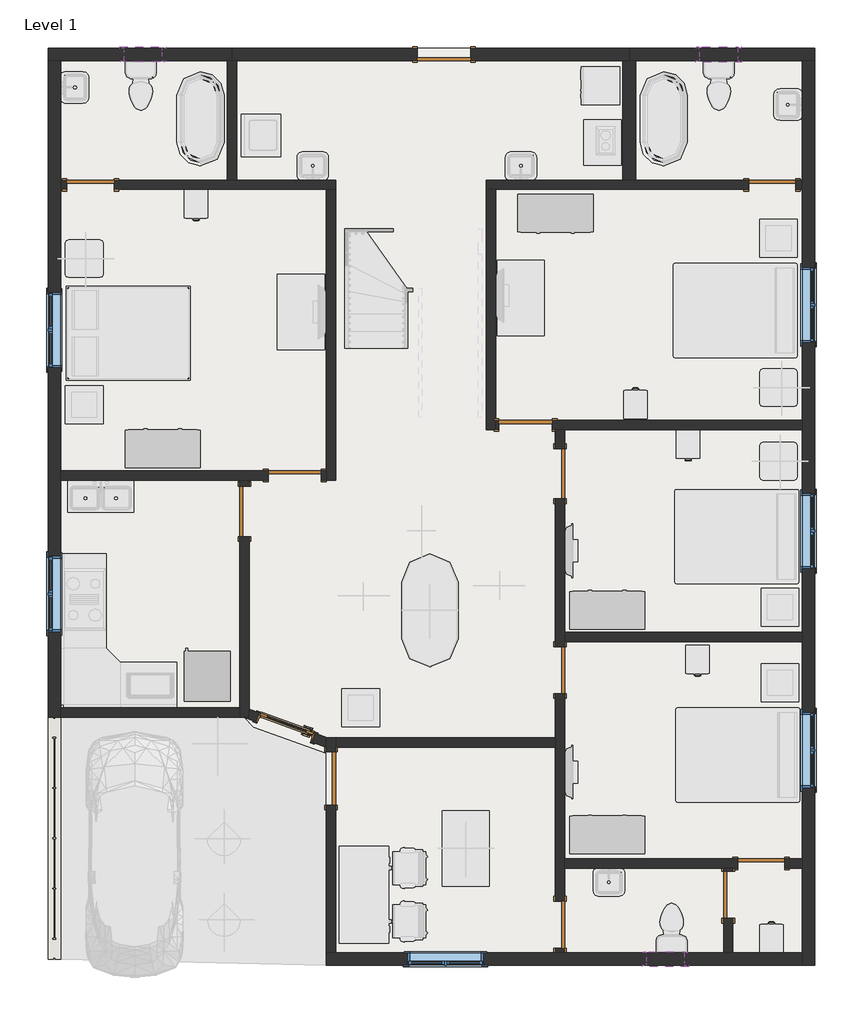
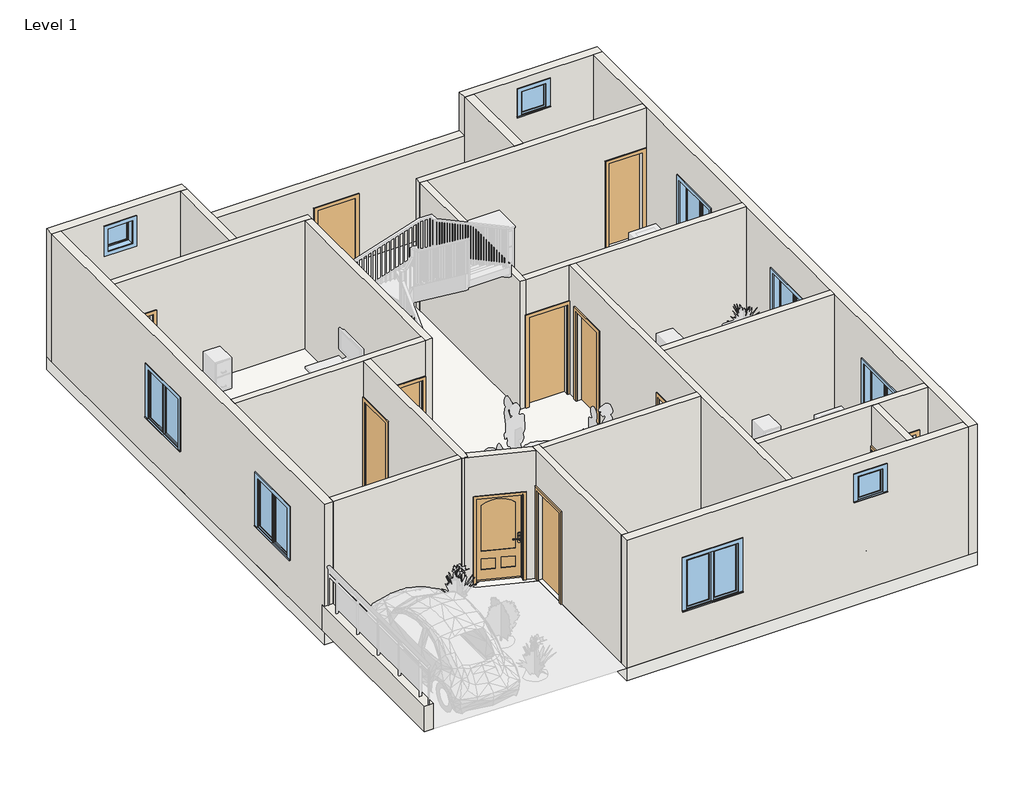
# One storey, part 1 of 3: 24 walls, 13 doors, 9 windows, 1 slab.
"""IFC4 building model written with IfcOpenShell, lengths in millimetres."""

from ifc_helpers import new_model, si_unit, frame, origin, origin_with_axes, place, context, project, spatial, polyline, outline, extrude, faceted_brep, transform, mapped, element, save
from components import door_808aeb8e, door_255cab33, door_059fdd7e, door_377e7377, door_bb092f7c, door_3e6ab620, door_b6e9fca3, door_99d96fc5, window_0862ab64, window_e41d21a6

model = new_model("IFC4")

# Units and contexts
model_context = context("Model", 3, world=origin())
ifc_project = project(units=[si_unit("LENGTHUNIT", "METRE", prefix="MILLI")], contexts=[model_context])

# Site, building, storey
site = spatial("IfcSite", under=ifc_project)
building = spatial("IfcBuilding", under=site)
storey = spatial("IfcBuildingStorey", under=building, Name="Level 1", Elevation=0.0)

# Doors
placement = place(None, origin())
door_shape = door_808aeb8e(model_context)
element("IfcDoor", 1, ObjectType="36\" x 80\"", at=placement, inside=storey, context=model_context, shape_type="MappedRepresentation", body=[
    mapped(door_shape, transform((-11135.4937633, 2943.8996558, 0.0), x_axis=(0.9396926207859074, -0.3420201433256715, 0.0), y_axis=(0.3420201433256715, 0.9396926207859074, 0.0), z_axis=(0.0, 0.0, 1.0))),
])
door_2_shape = door_255cab33(model_context)
element("IfcDoor", 2, ObjectType="Single-Flush : 30\" x 80\"", at=placement, inside=storey, context=model_context, shape_type="MappedRepresentation", body=[
    mapped(door_2_shape, transform((-14290.4744419, 11717.2452409, 0.0), x_axis=(-1.0, 0.0, 0.0), y_axis=(0.0, -1.0, 0.0), z_axis=(0.0, 0.0, 1.0))),
])
element("IfcDoor", 3, ObjectType="Single-Flush : 30\" x 80\"", at=placement, inside=storey, context=model_context, shape_type="MappedRepresentation", body=[
    mapped(door_2_shape, transform((-6695.8744419, 3868.6452409, 0.0), x_axis=(0.0, 1.0, 0.0), y_axis=(-1.0, 0.0, 0.0), z_axis=(0.0, 0.0, 1.0))),
])
element("IfcDoor", 4, ObjectType="Single-Flush : 30\" x 80\"", at=placement, inside=storey, context=model_context, shape_type="MappedRepresentation", body=[
    mapped(door_2_shape, transform((-3444.6744419, 744.4452409, 0.0), x_axis=(-1.0, 0.0, 0.0), y_axis=(0.0, -1.0, 0.0), z_axis=(0.0, 0.0, 1.0))),
])
door_3_shape = door_059fdd7e(model_context)
element("IfcDoor", 5, ObjectType="Single-Flush : 30\" x 80\"", at=placement, inside=storey, context=model_context, shape_type="MappedRepresentation", body=[
    mapped(door_3_shape, transform((-3266.8744419, 11717.2452409, 0.0), x_axis=(1.0, 0.0, 0.0), y_axis=(0.0, 1.0, 0.0), z_axis=(0.0, 0.0, 1.0))),
])
element("IfcDoor", 6, ObjectType="Single-Flush : 30\" x 80\"", at=placement, inside=storey, context=model_context, shape_type="MappedRepresentation", body=[
    mapped(door_3_shape, transform((-6695.8744419, -246.1547591, 0.0), x_axis=(0.0, -1.0, 0.0), y_axis=(1.0, 0.0, 0.0), z_axis=(0.0, 0.0, 1.0))),
])
element("IfcDoor", 7, ObjectType="Single-Flush : 30\" x 80\"", at=placement, inside=storey, context=model_context, shape_type="MappedRepresentation", body=[
    mapped(door_3_shape, transform((-3978.0744419, 236.4452409, 0.0), x_axis=(0.0, 1.0, 0.0), y_axis=(-1.0, 0.0, 0.0), z_axis=(0.0, 0.0, 1.0))),
])
door_4_shape = door_377e7377(model_context)
element("IfcDoor", 8, ObjectType="Single-Flush : 32\" x 84\"", at=placement, inside=storey, context=model_context, shape_type="MappedRepresentation", body=[
    mapped(door_4_shape, transform((-11801.2744419, 6434.0452409, 0.0), x_axis=(0.0, 1.0, 0.0), y_axis=(-1.0, 0.0, 0.0), z_axis=(0.0, 0.0, 1.0))),
])
door_5_shape = door_bb092f7c(model_context)
element("IfcDoor", 9, ObjectType="Single-Flush : 32\" x 84\"", at=placement, inside=storey, context=model_context, shape_type="MappedRepresentation", body=[
    mapped(door_5_shape, transform((-6695.8744419, 7043.6452409, 0.0), x_axis=(0.0, 1.0, 0.0), y_axis=(-1.0, 0.0, 0.0), z_axis=(0.0, 0.0, 1.0))),
])
door_6_shape = door_3e6ab620(model_context)
element("IfcDoor", 10, ObjectType="Single-Flush : 34\" x 60\"", at=placement, inside=storey, context=model_context, shape_type="MappedRepresentation", body=[
    mapped(door_6_shape, transform((-8575.4744419, 13825.4452409, 0.0), x_axis=(-1.0, 0.0, 0.0), y_axis=(0.0, -1.0, 0.0), z_axis=(0.0, 0.0, 1.0))),
])
door_7_shape = door_b6e9fca3(model_context)
element("IfcDoor", 11, ObjectType="Single-Flush : 34\" x 84\"", at=placement, inside=storey, context=model_context, shape_type="MappedRepresentation", body=[
    mapped(door_7_shape, transform((-10988.4744419, 7018.2452409, 0.0), x_axis=(1.0, 0.0, 0.0), y_axis=(0.0, 1.0, 0.0), z_axis=(0.0, 0.0, 1.0))),
])
door_8_shape = door_99d96fc5(model_context)
element("IfcDoor", 12, ObjectType="Single-Flush : 34\" x 84\"", at=placement, inside=storey, context=model_context, shape_type="MappedRepresentation", body=[
    mapped(door_8_shape, transform((-7254.6744419, 7831.0452409, 0.0), x_axis=(-1.0, 0.0, 0.0), y_axis=(0.0, -1.0, 0.0), z_axis=(0.0, 0.0, 1.0))),
])
element("IfcDoor", 13, ObjectType="Single-Flush : 34\" x 84\"", at=placement, inside=storey, context=model_context, shape_type="MappedRepresentation", body=[
    mapped(door_8_shape, transform((-10404.2744419, 2116.0452409, 0.0), x_axis=(0.0, 1.0, 0.0), y_axis=(-1.0, 0.0, 0.0), z_axis=(0.0, 0.0, 1.0))),
])

# Slab
element("IfcSlab", 14, ObjectType="Generic - 12\"", at=placement, inside=storey, context=model_context, shape_type="SweptSolid", body=[
    extrude(outline(polyline([(-2581.0744419, 13927.0452409), (-2581.0744419, -906.5547591), (-10480.4744419, -906.5547591), (-10480.4744419, 2522.4452409), (-11647.819555, 2947.3241152), (-11807.1406807, 3106.6452409), (-14976.2744419, 3106.6452409), (-14976.2744419, 13927.0452409), (-2581.0744419, 13927.0452409)])), frame((0.0, 0.0, -304.8), z_axis=(0.0, 0.0, 1.0), x_axis=(1.0, 0.0, 0.0)), (0.0, 0.0, 1.0), 304.8),
])

# Walls
element("IfcWall", 15, ObjectType="Generic - 2'", at=placement, inside=storey, context=model_context, shape_type="Brep", body=[
    faceted_brep([(-14773.0744419, -804.9547591, 0.0), (-14773.0744419, 3106.6452409, 0.0), (-14773.0744419, 3182.8452409, 0.0), (-14773.0744419, 3182.8452409, 609.6), (-14773.0744419, -804.9547591, 609.6), (-14976.2744419, -804.9547591, 0.0), (-14976.2744419, -804.9547591, 609.6), (-14976.2744419, 3182.8452409, 609.6), (-14976.2744419, 3182.8452409, 0.0)], [[[0, 1, 2, 3, 4]], [[5, 6, 7, 8]], [[2, 1, 0, 5, 8]], [[3, 2, 8, 7]], [[4, 3, 7, 6]], [[0, 4, 6, 5]]]),
])
element("IfcWall", 16, ObjectType="Generic - 8\"", at=placement, inside=storey, context=model_context, shape_type="Brep", body=[
    faceted_brep([(-14976.2744419, 13723.8452409, 0.0), (-14773.0744419, 13723.8452409, 0.0), (-12080.6744419, 13723.8452409, 0.0), (-12004.4744419, 13723.8452409, 0.0), (-12004.4744419, 13723.8452409, 2133.6), (-11928.2744419, 13723.8452409, 2133.6), (-11928.2744419, 13723.8452409, 3048.0), (-12080.6744419, 13723.8452409, 3048.0), (-14773.0744419, 13723.8452409, 3048.0), (-14976.2744419, 13723.8452409, 3048.0), (-13134.7744419, 13723.8452409, 2768.6), (-13134.7744419, 13723.8452409, 2159.0), (-13744.3744419, 13723.8452409, 2159.0), (-13744.3744419, 13723.8452409, 2768.6), (-14976.2744419, 13927.0452409, 0.0), (-14976.2744419, 13927.0452409, 3048.0), (-11928.2744419, 13927.0452409, 3048.0), (-11928.2744419, 13927.0452409, 2133.6), (-12004.4744419, 13927.0452409, 2133.6), (-12004.4744419, 13927.0452409, 0.0), (-13134.7744419, 13927.0452409, 2768.6), (-13744.3744419, 13927.0452409, 2768.6), (-13744.3744419, 13927.0452409, 2159.0), (-13134.7744419, 13927.0452409, 2159.0)], [[[0, 1, 2, 3, 4, 5, 6, 7, 8, 9], [10, 11, 12, 13]], [[14, 15, 16, 17, 18, 19], [20, 21, 22, 23]], [[3, 2, 1, 0, 14, 19]], [[0, 9, 15, 14]], [[11, 10, 20, 23]], [[12, 11, 23, 22]], [[13, 12, 22, 21]], [[10, 13, 21, 20]], [[4, 3, 19, 18]], [[17, 5, 4, 18]], [[6, 5, 17, 16]], [[9, 8, 7, 6, 16, 15]]]),
])
element("IfcWall", 17, ObjectType="Generic - 8\"", at=placement, inside=storey, context=model_context, shape_type="Brep", body=[
    faceted_brep([(-2784.2744419, 13723.8452409, 0.0), (-2784.2744419, 11793.4452409, 0.0), (-2784.2744419, 11641.0452409, 0.0), (-2784.2744419, 7907.2452409, 0.0), (-2784.2744419, 7754.8452409, 0.0), (-2784.2744419, 4478.2452409, 0.0), (-2784.2744419, 4325.8452409, 0.0), (-2784.2744419, 820.6452409, 0.0), (-2784.2744419, 668.2452409, 0.0), (-2784.2744419, -703.3547591, 0.0), (-2784.2744419, -906.5547591, 0.0), (-2784.2744419, -906.5547591, 3048.0), (-2784.2744419, -703.3547591, 3048.0), (-2784.2744419, 668.2452409, 3048.0), (-2784.2744419, 820.6452409, 3048.0), (-2784.2744419, 4325.8452409, 3048.0), (-2784.2744419, 4478.2452409, 3048.0), (-2784.2744419, 7754.8452409, 3048.0), (-2784.2744419, 7907.2452409, 3048.0), (-2784.2744419, 11641.0452409, 3048.0), (-2784.2744419, 11793.4452409, 3048.0), (-2784.2744419, 13723.8452409, 3048.0), (-2784.2744419, 1963.6452409, 2133.6), (-2784.2744419, 1963.6452409, 914.4), (-2784.2744419, 3182.8452409, 914.4), (-2784.2744419, 3182.8452409, 2133.6), (-2784.2744419, 5506.9452409, 2133.6), (-2784.2744419, 5506.9452409, 914.4), (-2784.2744419, 6726.1452409, 914.4), (-2784.2744419, 6726.1452409, 2133.6), (-2784.2744419, 9164.5452409, 2133.6), (-2784.2744419, 9164.5452409, 914.4), (-2784.2744419, 10383.7452409, 914.4), (-2784.2744419, 10383.7452409, 2133.6), (-2581.0744419, 13723.8452409, 0.0), (-2581.0744419, 13723.8452409, 3048.0), (-2581.0744419, -906.5547591, 3048.0), (-2581.0744419, -906.5547591, 0.0), (-2581.0744419, 1963.6452409, 2133.6), (-2581.0744419, 3182.8452409, 2133.6), (-2581.0744419, 3182.8452409, 914.4), (-2581.0744419, 1963.6452409, 914.4), (-2581.0744419, 5506.9452409, 2133.6), (-2581.0744419, 6726.1452409, 2133.6), (-2581.0744419, 6726.1452409, 914.4), (-2581.0744419, 5506.9452409, 914.4), (-2581.0744419, 9164.5452409, 2133.6), (-2581.0744419, 10383.7452409, 2133.6), (-2581.0744419, 10383.7452409, 914.4), (-2581.0744419, 9164.5452409, 914.4)], [[[0, 1, 2, 3, 4, 5, 6, 7, 8, 9, 10, 11, 12, 13, 14, 15, 16, 17, 18, 19, 20, 21], [22, 23, 24, 25], [26, 27, 28, 29], [30, 31, 32, 33]], [[34, 35, 36, 37], [38, 39, 40, 41], [42, 43, 44, 45], [46, 47, 48, 49]], [[10, 9, 8, 7, 6, 5, 4, 3, 2, 1, 0, 34, 37]], [[0, 21, 35, 34]], [[11, 10, 37, 36]], [[23, 22, 38, 41]], [[24, 23, 41, 40]], [[25, 24, 40, 39]], [[22, 25, 39, 38]], [[27, 26, 42, 45]], [[28, 27, 45, 44]], [[29, 28, 44, 43]], [[26, 29, 43, 42]], [[31, 30, 46, 49]], [[32, 31, 49, 48]], [[33, 32, 48, 47]], [[30, 33, 47, 46]], [[21, 20, 19, 18, 17, 16, 15, 14, 13, 12, 11, 36, 35]]]),
])
element("IfcWall", 18, ObjectType="Generic - 8\"", at=placement, inside=storey, context=model_context, shape_type="Brep", body=[
    faceted_brep([(-2784.2744419, -703.3547591, 0.0), (-3901.8744419, -703.3547591, 0.0), (-4054.2744419, -703.3547591, 0.0), (-6619.6744419, -703.3547591, 0.0), (-6772.0744419, -703.3547591, 0.0), (-10328.0744419, -703.3547591, 0.0), (-10480.4744419, -703.3547591, 0.0), (-10480.4744419, -703.3547591, 3048.0), (-10328.0744419, -703.3547591, 3048.0), (-6772.0744419, -703.3547591, 3048.0), (-6619.6744419, -703.3547591, 3048.0), (-4054.2744419, -703.3547591, 3048.0), (-3901.8744419, -703.3547591, 3048.0), (-2784.2744419, -703.3547591, 3048.0), (-9159.6744419, -703.3547591, 2133.6), (-9159.6744419, -703.3547591, 914.4), (-7940.4744419, -703.3547591, 914.4), (-7940.4744419, -703.3547591, 2133.6), (-5298.8744419, -703.3547591, 2768.6), (-5298.8744419, -703.3547591, 2159.0), (-4689.2744419, -703.3547591, 2159.0), (-4689.2744419, -703.3547591, 2768.6), (-2784.2744419, -906.5547591, 0.0), (-2784.2744419, -906.5547591, 3048.0), (-10480.4744419, -906.5547591, 3048.0), (-10480.4744419, -906.5547591, 0.0), (-9159.6744419, -906.5547591, 2133.6), (-7940.4744419, -906.5547591, 2133.6), (-7940.4744419, -906.5547591, 914.4), (-9159.6744419, -906.5547591, 914.4), (-5298.8744419, -906.5547591, 2768.6), (-4689.2744419, -906.5547591, 2768.6), (-4689.2744419, -906.5547591, 2159.0), (-5298.8744419, -906.5547591, 2159.0)], [[[0, 1, 2, 3, 4, 5, 6, 7, 8, 9, 10, 11, 12, 13], [14, 15, 16, 17], [18, 19, 20, 21]], [[22, 23, 24, 25], [26, 27, 28, 29], [30, 31, 32, 33]], [[6, 5, 4, 3, 2, 1, 0, 22, 25]], [[0, 13, 23, 22]], [[15, 14, 26, 29]], [[16, 15, 29, 28]], [[17, 16, 28, 27]], [[14, 17, 27, 26]], [[19, 18, 30, 33]], [[20, 19, 33, 32]], [[21, 20, 32, 31]], [[18, 21, 31, 30]], [[7, 6, 25, 24]], [[13, 12, 11, 10, 9, 8, 7, 24, 23]]]),
])
element("IfcWall", 19, ObjectType="Generic - 8\"", at=placement, inside=storey, context=model_context, shape_type="Brep", body=[
    faceted_brep([(-5679.8744419, 13723.8452409, 3048.0), (-5679.8744419, 13723.8452409, 2133.6), (-5679.8744419, 13723.8452409, 0.0), (-5679.8744419, 11793.4452409, 0.0), (-5679.8744419, 11793.4452409, 3048.0), (-5476.6744419, 13723.8452409, 0.0), (-5476.6744419, 13723.8452409, 3048.0), (-5476.6744419, 11793.4452409, 3048.0), (-5476.6744419, 11793.4452409, 0.0), (-5578.2744419, 13723.8452409, 0.0)], [[[0, 1, 2, 3, 4]], [[5, 6, 7, 8]], [[3, 2, 9, 5, 8]], [[4, 3, 8, 7]], [[0, 6, 5, 9, 2, 1]], [[0, 4, 7, 6]]]),
])
element("IfcWall", 20, ObjectType="Generic - 8\"", at=placement, inside=storey, context=model_context, shape_type="Brep", body=[
    faceted_brep([(-5578.2744419, 13723.8452409, 0.0), (-5578.2744419, 13723.8452409, 2133.6), (-5679.8744419, 13723.8452409, 2133.6), (-11928.2744419, 13723.8452409, 2133.6), (-12004.4744419, 13723.8452409, 2133.6), (-12004.4744419, 13723.8452409, 0.0), (-11928.2744419, 13723.8452409, 0.0), (-9007.2744419, 13723.8452409, 0.0), (-9007.2744419, 13723.8452409, 1524.0), (-8143.6744419, 13723.8452409, 1524.0), (-8143.6744419, 13723.8452409, 0.0), (-5679.8744419, 13723.8452409, 0.0), (-5578.2744419, 13927.0452409, 2133.6), (-5578.2744419, 13927.0452409, 0.0), (-8143.6744419, 13927.0452409, 0.0), (-8143.6744419, 13927.0452409, 1524.0), (-9007.2744419, 13927.0452409, 1524.0), (-9007.2744419, 13927.0452409, 0.0), (-12004.4744419, 13927.0452409, 0.0), (-12004.4744419, 13927.0452409, 2133.6), (-11928.2744419, 13927.0452409, 2133.6), (-5679.8744419, 13927.0452409, 2133.6)], [[[0, 1, 2, 3, 4, 5, 6, 7, 8, 9, 10, 11]], [[12, 13, 14, 15, 16, 17, 18, 19, 20, 21]], [[5, 18, 17, 7, 6]], [[13, 0, 11, 10, 14]], [[1, 0, 13, 12]], [[4, 3, 2, 1, 12, 21, 20, 19]], [[5, 4, 19, 18]], [[16, 8, 7, 17]], [[9, 15, 14, 10]], [[15, 9, 8, 16]]]),
])
element("IfcWall", 21, ObjectType="Generic - 8\"", at=placement, inside=storey, context=model_context, shape_type="Brep", body=[
    faceted_brep([(-5578.2744419, 13723.8452409, 0.0), (-5476.6744419, 13723.8452409, 0.0), (-2784.2744419, 13723.8452409, 0.0), (-2581.0744419, 13723.8452409, 0.0), (-2581.0744419, 13723.8452409, 3048.0), (-2784.2744419, 13723.8452409, 3048.0), (-5476.6744419, 13723.8452409, 3048.0), (-5679.8744419, 13723.8452409, 3048.0), (-5679.8744419, 13723.8452409, 2133.6), (-5578.2744419, 13723.8452409, 2133.6), (-4435.2744419, 13723.8452409, 2768.6), (-3825.6744419, 13723.8452409, 2768.6), (-3825.6744419, 13723.8452409, 2159.0), (-4435.2744419, 13723.8452409, 2159.0), (-5578.2744419, 13927.0452409, 0.0), (-5578.2744419, 13927.0452409, 2133.6), (-5679.8744419, 13927.0452409, 2133.6), (-5679.8744419, 13927.0452409, 3048.0), (-2581.0744419, 13927.0452409, 3048.0), (-2581.0744419, 13927.0452409, 0.0), (-4435.2744419, 13927.0452409, 2768.6), (-4435.2744419, 13927.0452409, 2159.0), (-3825.6744419, 13927.0452409, 2159.0), (-3825.6744419, 13927.0452409, 2768.6)], [[[0, 1, 2, 3, 4, 5, 6, 7, 8, 9], [10, 11, 12, 13]], [[14, 15, 16, 17, 18, 19], [20, 21, 22, 23]], [[3, 2, 1, 0, 14, 19]], [[4, 3, 19, 18]], [[20, 23, 11, 10]], [[23, 22, 12, 11]], [[22, 21, 13, 12]], [[21, 20, 10, 13]], [[0, 9, 15, 14]], [[8, 16, 15, 9]], [[8, 7, 17, 16]], [[7, 6, 5, 4, 18, 17]]]),
])
element("IfcWall", 22, ObjectType="Generic - 8\"", at=placement, inside=storey, context=model_context, shape_type="Brep", body=[
    faceted_brep([(-14773.0744419, 3182.8452409, 0.0), (-14773.0744419, 3259.0452409, 0.0), (-14773.0744419, 6942.0452409, 0.0), (-14773.0744419, 7094.4452409, 0.0), (-14773.0744419, 11641.0452409, 0.0), (-14773.0744419, 11793.4452409, 0.0), (-14773.0744419, 13723.8452409, 0.0), (-14773.0744419, 13723.8452409, 3048.0), (-14773.0744419, 11793.4452409, 3048.0), (-14773.0744419, 11641.0452409, 3048.0), (-14773.0744419, 7094.4452409, 3048.0), (-14773.0744419, 6942.0452409, 3048.0), (-14773.0744419, 3259.0452409, 3048.0), (-14773.0744419, 3106.6452409, 3048.0), (-14773.0744419, 3106.6452409, 609.6), (-14773.0744419, 3182.8452409, 609.6), (-14773.0744419, 9977.3452409, 2133.6), (-14773.0744419, 9977.3452409, 914.4), (-14773.0744419, 8758.1452409, 914.4), (-14773.0744419, 8758.1452409, 2133.6), (-14773.0744419, 5710.1452409, 2133.6), (-14773.0744419, 5710.1452409, 914.4), (-14773.0744419, 4490.9452409, 914.4), (-14773.0744419, 4490.9452409, 2133.6), (-14976.2744419, 3182.8452409, 0.0), (-14976.2744419, 3182.8452409, 609.6), (-14976.2744419, 3106.6452409, 609.6), (-14976.2744419, 3106.6452409, 3048.0), (-14976.2744419, 13723.8452409, 3048.0), (-14976.2744419, 13723.8452409, 0.0), (-14976.2744419, 9977.3452409, 2133.6), (-14976.2744419, 8758.1452409, 2133.6), (-14976.2744419, 8758.1452409, 914.4), (-14976.2744419, 9977.3452409, 914.4), (-14976.2744419, 5710.1452409, 2133.6), (-14976.2744419, 4490.9452409, 2133.6), (-14976.2744419, 4490.9452409, 914.4), (-14976.2744419, 5710.1452409, 914.4)], [[[0, 1, 2, 3, 4, 5, 6, 7, 8, 9, 10, 11, 12, 13, 14, 15], [16, 17, 18, 19], [20, 21, 22, 23]], [[24, 25, 26, 27, 28, 29], [30, 31, 32, 33], [34, 35, 36, 37]], [[6, 5, 4, 3, 2, 1, 0, 24, 29]], [[7, 6, 29, 28]], [[16, 19, 31, 30]], [[19, 18, 32, 31]], [[18, 17, 33, 32]], [[17, 16, 30, 33]], [[20, 23, 35, 34]], [[23, 22, 36, 35]], [[22, 21, 37, 36]], [[21, 20, 34, 37]], [[0, 15, 25, 24]], [[14, 26, 25, 15]], [[14, 13, 27, 26]], [[13, 12, 11, 10, 9, 8, 7, 28, 27]]]),
])
element("IfcWall", 23, ObjectType="INNER 6\"", at=placement, inside=storey, context=model_context, shape_type="Brep", body=[
    faceted_brep([(-14773.0744419, 11641.0452409, 0.0), (-14671.4744419, 11641.0452409, 0.0), (-14671.4744419, 11641.0452409, 2032.0), (-13909.4744419, 11641.0452409, 2032.0), (-13909.4744419, 11641.0452409, 0.0), (-10480.4744419, 11641.0452409, 0.0), (-10328.0744419, 11641.0452409, 0.0), (-10328.0744419, 11641.0452409, 3048.0), (-10480.4744419, 11641.0452409, 3048.0), (-14773.0744419, 11641.0452409, 3048.0), (-14671.4744419, 11793.4452409, 2032.0), (-14671.4744419, 11793.4452409, 0.0), (-14773.0744419, 11793.4452409, 0.0), (-14773.0744419, 11793.4452409, 3048.0), (-12080.6744419, 11793.4452409, 3048.0), (-11928.2744419, 11793.4452409, 3048.0), (-10328.0744419, 11793.4452409, 3048.0), (-10328.0744419, 11793.4452409, 0.0), (-11928.2744419, 11793.4452409, 0.0), (-12080.6744419, 11793.4452409, 0.0), (-13909.4744419, 11793.4452409, 0.0), (-13909.4744419, 11793.4452409, 2032.0)], [[[0, 1, 2, 3, 4, 5, 6, 7, 8, 9]], [[10, 11, 12, 13, 14, 15, 16, 17, 18, 19, 20, 21]], [[12, 11, 1, 0]], [[20, 19, 18, 17, 6, 5, 4]], [[0, 9, 13, 12]], [[2, 1, 11, 10]], [[3, 2, 10, 21]], [[4, 3, 21, 20]], [[7, 6, 17, 16]], [[9, 8, 7, 16, 15, 14, 13]]]),
])
element("IfcWall", 24, ObjectType="INNER 6\"", at=placement, inside=storey, context=model_context, shape_type="Brep", body=[
    faceted_brep([(-12080.6744419, 13723.8452409, 3048.0), (-12080.6744419, 13723.8452409, 0.0), (-12080.6744419, 11793.4452409, 0.0), (-12080.6744419, 11793.4452409, 3048.0), (-11928.2744419, 13723.8452409, 0.0), (-11928.2744419, 13723.8452409, 2133.6), (-11928.2744419, 13723.8452409, 3048.0), (-11928.2744419, 11793.4452409, 3048.0), (-11928.2744419, 11793.4452409, 0.0), (-12004.4744419, 13723.8452409, 0.0)], [[[0, 1, 2, 3]], [[4, 5, 6, 7, 8]], [[2, 1, 9, 4, 8]], [[3, 2, 8, 7]], [[0, 6, 5, 4, 9, 1]], [[0, 3, 7, 6]]]),
])
element("IfcWall", 25, ObjectType="INNER 6\"", at=placement, inside=storey, context=model_context, shape_type="Brep", body=[
    faceted_brep([(-10480.4744419, 11641.0452409, 0.0), (-10480.4744419, 7094.4452409, 0.0), (-10480.4744419, 6942.0452409, 0.0), (-10480.4744419, 6942.0452409, 3048.0), (-10480.4744419, 7094.4452409, 3048.0), (-10480.4744419, 11641.0452409, 3048.0), (-10328.0744419, 11641.0452409, 0.0), (-10328.0744419, 11641.0452409, 3048.0), (-10328.0744419, 6942.0452409, 3048.0), (-10328.0744419, 6942.0452409, 0.0)], [[[0, 1, 2, 3, 4, 5]], [[6, 7, 8, 9]], [[2, 1, 0, 6, 9]], [[0, 5, 7, 6]], [[3, 2, 9, 8]], [[5, 4, 3, 8, 7]]]),
])
element("IfcWall", 26, ObjectType="INNER 6\"", at=placement, inside=storey, context=model_context, shape_type="Brep", body=[
    faceted_brep([(-10480.4744419, 7094.4452409, 0.0), (-10556.6744419, 7094.4452409, 0.0), (-10556.6744419, 7094.4452409, 2133.6), (-11420.2744419, 7094.4452409, 2133.6), (-11420.2744419, 7094.4452409, 0.0), (-14773.0744419, 7094.4452409, 0.0), (-14773.0744419, 7094.4452409, 3048.0), (-10480.4744419, 7094.4452409, 3048.0), (-10556.6744419, 6942.0452409, 2133.6), (-10556.6744419, 6942.0452409, 0.0), (-10480.4744419, 6942.0452409, 0.0), (-10480.4744419, 6942.0452409, 3048.0), (-11725.0744419, 6942.0452409, 3048.0), (-11877.4744419, 6942.0452409, 3048.0), (-14773.0744419, 6942.0452409, 3048.0), (-14773.0744419, 6942.0452409, 0.0), (-11877.4744419, 6942.0452409, 0.0), (-11725.0744419, 6942.0452409, 0.0), (-11420.2744419, 6942.0452409, 0.0), (-11420.2744419, 6942.0452409, 2133.6)], [[[0, 1, 2, 3, 4, 5, 6, 7]], [[8, 9, 10, 11, 12, 13, 14, 15, 16, 17, 18, 19]], [[10, 9, 1, 0]], [[18, 17, 16, 15, 5, 4]], [[0, 7, 11, 10]], [[6, 5, 15, 14]], [[2, 1, 9, 8]], [[3, 2, 8, 19]], [[4, 3, 19, 18]], [[7, 6, 14, 13, 12, 11]]]),
])
element("IfcWall", 27, ObjectType="INNER 6\"", at=placement, inside=storey, context=model_context, shape_type="Brep", body=[
    faceted_brep([(-7889.6744419, 11641.0452409, 0.0), (-7889.6744419, 7754.8452409, 0.0), (-7889.6744419, 7754.8452409, 3048.0), (-7889.6744419, 11641.0452409, 3048.0), (-7737.2744419, 11641.0452409, 0.0), (-7737.2744419, 11641.0452409, 3048.0), (-7737.2744419, 7907.2452409, 3048.0), (-7737.2744419, 7754.8452409, 3048.0), (-7737.2744419, 7754.8452409, 0.0), (-7737.2744419, 7907.2452409, 0.0)], [[[0, 1, 2, 3]], [[4, 5, 6, 7, 8, 9]], [[1, 0, 4, 9, 8]], [[0, 3, 5, 4]], [[2, 1, 8, 7]], [[3, 2, 7, 6, 5]]]),
])
element("IfcWall", 28, ObjectType="INNER 6\"", at=placement, inside=storey, context=model_context, shape_type="Brep", body=[
    faceted_brep([(-7737.2744419, 7754.8452409, 3048.0), (-7737.2744419, 7754.8452409, 0.0), (-7686.4744419, 7754.8452409, 0.0), (-7686.4744419, 7754.8452409, 2133.6), (-6822.8744419, 7754.8452409, 2133.6), (-6822.8744419, 7754.8452409, 0.0), (-6772.0744419, 7754.8452409, 0.0), (-6619.6744419, 7754.8452409, 0.0), (-2784.2744419, 7754.8452409, 0.0), (-2784.2744419, 7754.8452409, 3048.0), (-6619.6744419, 7754.8452409, 3048.0), (-6772.0744419, 7754.8452409, 3048.0), (-7737.2744419, 7907.2452409, 0.0), (-7737.2744419, 7907.2452409, 3048.0), (-2784.2744419, 7907.2452409, 3048.0), (-2784.2744419, 7907.2452409, 0.0), (-6822.8744419, 7907.2452409, 0.0), (-6822.8744419, 7907.2452409, 2133.6), (-7686.4744419, 7907.2452409, 2133.6), (-7686.4744419, 7907.2452409, 0.0)], [[[0, 1, 2, 3, 4, 5, 6, 7, 8, 9, 10, 11]], [[12, 13, 14, 15, 16, 17, 18, 19]], [[1, 12, 19, 2]], [[15, 8, 7, 6, 5, 16]], [[1, 0, 13, 12]], [[9, 8, 15, 14]], [[18, 3, 2, 19]], [[3, 18, 17, 4]], [[4, 17, 16, 5]], [[0, 11, 10, 9, 14, 13]]]),
])
element("IfcWall", 29, ObjectType="INNER 6\"", at=placement, inside=storey, context=model_context, shape_type="Brep", body=[
    faceted_brep([(-11877.4744419, 6942.0452409, 0.0), (-11877.4744419, 6840.4452409, 0.0), (-11877.4744419, 6840.4452409, 2133.6), (-11877.4744419, 6027.6452409, 2133.6), (-11877.4744419, 6027.6452409, 0.0), (-11877.4744419, 3259.0452409, 0.0), (-11877.4744419, 3106.6452409, 0.0), (-11877.4744419, 3106.6452409, 3048.0), (-11877.4744419, 3259.0452409, 3048.0), (-11877.4744419, 6942.0452409, 3048.0), (-11725.0744419, 6840.4452409, 2133.6), (-11725.0744419, 6840.4452409, 0.0), (-11725.0744419, 6942.0452409, 0.0), (-11725.0744419, 6942.0452409, 3048.0), (-11725.0744419, 3236.2010554, 3048.0), (-11725.0744419, 3106.6452409, 3048.0), (-11725.0744419, 3106.6452409, 0.0), (-11725.0744419, 3236.2010554, 0.0), (-11725.0744419, 6027.6452409, 0.0), (-11725.0744419, 6027.6452409, 2133.6), (-11814.7105578, 3106.6452409, 0.0), (-11807.1406807, 3106.6452409, 3048.0), (-11814.7105578, 3106.6452409, 3048.0)], [[[0, 1, 2, 3, 4, 5, 6, 7, 8, 9]], [[10, 11, 12, 13, 14, 15, 16, 17, 18, 19]], [[12, 11, 1, 0]], [[18, 17, 16, 20, 6, 5, 4]], [[0, 9, 13, 12]], [[7, 6, 20, 16, 15, 21, 22]], [[2, 1, 11, 10]], [[3, 2, 10, 19]], [[4, 3, 19, 18]], [[9, 8, 7, 22, 21, 15, 14, 13]]]),
])
element("IfcWall", 30, ObjectType="INNER 6\"", at=placement, inside=storey, context=model_context, shape_type="Brep", body=[
    faceted_brep([(-11877.4744419, 3259.0452409, 0.0), (-14773.0744419, 3259.0452409, 0.0), (-14773.0744419, 3259.0452409, 3048.0), (-11877.4744419, 3259.0452409, 3048.0), (-11877.4744419, 3106.6452409, 0.0), (-11877.4744419, 3106.6452409, 3048.0), (-14773.0744419, 3106.6452409, 3048.0), (-14773.0744419, 3106.6452409, 609.6), (-14773.0744419, 3106.6452409, 0.0), (-14773.0744419, 3182.8452409, 0.0)], [[[0, 1, 2, 3]], [[4, 5, 6, 7, 8]], [[1, 0, 4, 8, 9]], [[0, 3, 5, 4]], [[1, 9, 8, 7, 6, 2]], [[3, 2, 6, 5]]]),
])
element("IfcWall", 31, ObjectType="INNER 6\"", at=placement, inside=storey, context=model_context, shape_type="SweptSolid", body=[
    extrude(outline(polyline([(-2784.2744419, 4325.8452409), (-6619.6744419, 4325.8452409), (-6619.6744419, 4478.2452409), (-2784.2744419, 4478.2452409), (-2784.2744419, 4325.8452409)])), origin_with_axes(), (0.0, 0.0, 1.0), 3048.0),
])
element("IfcWall", 32, ObjectType="INNER 6\"", at=placement, inside=storey, context=model_context, shape_type="Brep", body=[
    faceted_brep([(-10480.4744419, -703.3547591, 0.0), (-10480.4744419, -703.3547591, 3048.0), (-10480.4744419, 2522.4452409, 3048.0), (-10480.4744419, 2621.0230093, 3048.0), (-10480.4744419, 2776.4452409, 3048.0), (-10480.4744419, 2776.4452409, 0.0), (-10480.4744419, 2621.0230093, 0.0), (-10480.4744419, 2547.8452409, 0.0), (-10480.4744419, 2547.8452409, 2133.6), (-10480.4744419, 1684.2452409, 2133.6), (-10480.4744419, 1684.2452409, 0.0), (-10328.0744419, 2776.4452409, 3048.0), (-10328.0744419, 2624.0452409, 3048.0), (-10328.0744419, -703.3547591, 3048.0), (-10328.0744419, -703.3547591, 0.0), (-10328.0744419, 1684.2452409, 0.0), (-10328.0744419, 1684.2452409, 2133.6), (-10328.0744419, 2547.8452409, 2133.6), (-10328.0744419, 2547.8452409, 0.0), (-10328.0744419, 2624.0452409, 0.0), (-10328.0744419, 2776.4452409, 0.0), (-10461.9057233, 2776.4452409, 0.0), (-10461.9057233, 2776.4452409, 3048.0)], [[[0, 1, 2, 3, 4, 5, 6, 7, 8, 9, 10]], [[11, 12, 13, 14, 15, 16, 17, 18, 19, 20]], [[14, 0, 10, 15]], [[5, 21, 20, 19, 18, 7, 6]], [[1, 0, 14, 13]], [[5, 4, 22, 11, 20, 21]], [[8, 17, 16, 9]], [[9, 16, 15, 10]], [[17, 8, 7, 18]], [[13, 12, 11, 22, 4, 3, 2, 1]]]),
])
element("IfcWall", 33, ObjectType="INNER 6\"", at=placement, inside=storey, context=model_context, shape_type="Brep", body=[
    faceted_brep([(-6619.6744419, 668.2452409, 0.0), (-4054.2744419, 668.2452409, 0.0), (-3901.8744419, 668.2452409, 0.0), (-3825.6744419, 668.2452409, 0.0), (-3825.6744419, 668.2452409, 2032.0), (-3063.6744419, 668.2452409, 2032.0), (-3063.6744419, 668.2452409, 0.0), (-2784.2744419, 668.2452409, 0.0), (-2784.2744419, 668.2452409, 3048.0), (-3901.8744419, 668.2452409, 3048.0), (-4054.2744419, 668.2452409, 3048.0), (-6619.6744419, 668.2452409, 3048.0), (-3825.6744419, 820.6452409, 2032.0), (-3825.6744419, 820.6452409, 0.0), (-6619.6744419, 820.6452409, 0.0), (-6619.6744419, 820.6452409, 3048.0), (-2784.2744419, 820.6452409, 3048.0), (-2784.2744419, 820.6452409, 0.0), (-3063.6744419, 820.6452409, 0.0), (-3063.6744419, 820.6452409, 2032.0)], [[[0, 1, 2, 3, 4, 5, 6, 7, 8, 9, 10, 11]], [[12, 13, 14, 15, 16, 17, 18, 19]], [[18, 17, 7, 6]], [[14, 13, 3, 2, 1, 0]], [[8, 7, 17, 16]], [[0, 11, 15, 14]], [[4, 3, 13, 12]], [[5, 4, 12, 19]], [[6, 5, 19, 18]], [[11, 10, 9, 8, 16, 15]]]),
])
element("IfcWall", 34, ObjectType="INNER 6\"", at=placement, inside=storey, context=model_context, shape_type="Brep", body=[
    faceted_brep([(-2885.8744419, 11641.0452409, 2032.0), (-2885.8744419, 11641.0452409, 0.0), (-2784.2744419, 11641.0452409, 0.0), (-2784.2744419, 11641.0452409, 3048.0), (-7737.2744419, 11641.0452409, 3048.0), (-7889.6744419, 11641.0452409, 3048.0), (-7889.6744419, 11641.0452409, 0.0), (-7737.2744419, 11641.0452409, 0.0), (-3647.8744419, 11641.0452409, 0.0), (-3647.8744419, 11641.0452409, 2032.0), (-2784.2744419, 11793.4452409, 0.0), (-2885.8744419, 11793.4452409, 0.0), (-2885.8744419, 11793.4452409, 2032.0), (-3647.8744419, 11793.4452409, 2032.0), (-3647.8744419, 11793.4452409, 0.0), (-5476.6744419, 11793.4452409, 0.0), (-5679.8744419, 11793.4452409, 0.0), (-7889.6744419, 11793.4452409, 0.0), (-7889.6744419, 11793.4452409, 3048.0), (-5679.8744419, 11793.4452409, 3048.0), (-5476.6744419, 11793.4452409, 3048.0), (-2784.2744419, 11793.4452409, 3048.0)], [[[0, 1, 2, 3, 4, 5, 6, 7, 8, 9]], [[10, 11, 12, 13, 14, 15, 16, 17, 18, 19, 20, 21]], [[2, 1, 11, 10]], [[8, 7, 6, 17, 16, 15, 14]], [[3, 2, 10, 21]], [[6, 5, 18, 17]], [[12, 11, 1, 0]], [[13, 12, 0, 9]], [[14, 13, 9, 8]], [[5, 4, 3, 21, 20, 19, 18]]]),
])
element("IfcWall", 35, ObjectType="INNER 6\"", at=placement, inside=storey, context=model_context, shape_type="Brep", body=[
    faceted_brep([(-6772.0744419, -627.1547591, 2032.0), (-6772.0744419, -627.1547591, 0.0), (-6772.0744419, -703.3547591, 0.0), (-6772.0744419, -703.3547591, 3048.0), (-6772.0744419, 2624.0452409, 3048.0), (-6772.0744419, 2776.4452409, 3048.0), (-6772.0744419, 7754.8452409, 3048.0), (-6772.0744419, 7754.8452409, 0.0), (-6772.0744419, 7450.0452409, 0.0), (-6772.0744419, 7450.0452409, 2133.6), (-6772.0744419, 6637.2452409, 2133.6), (-6772.0744419, 6637.2452409, 0.0), (-6772.0744419, 4249.6452409, 0.0), (-6772.0744419, 4249.6452409, 2032.0), (-6772.0744419, 3487.6452409, 2032.0), (-6772.0744419, 3487.6452409, 0.0), (-6772.0744419, 2776.4452409, 0.0), (-6772.0744419, 2624.0452409, 0.0), (-6772.0744419, 134.8452409, 0.0), (-6772.0744419, 134.8452409, 2032.0), (-6619.6744419, -703.3547591, 0.0), (-6619.6744419, -627.1547591, 0.0), (-6619.6744419, -627.1547591, 2032.0), (-6619.6744419, 134.8452409, 2032.0), (-6619.6744419, 134.8452409, 0.0), (-6619.6744419, 668.2452409, 0.0), (-6619.6744419, 820.6452409, 0.0), (-6619.6744419, 3487.6452409, 0.0), (-6619.6744419, 3487.6452409, 2032.0), (-6619.6744419, 4249.6452409, 2032.0), (-6619.6744419, 4249.6452409, 0.0), (-6619.6744419, 4325.8452409, 0.0), (-6619.6744419, 4478.2452409, 0.0), (-6619.6744419, 6637.2452409, 0.0), (-6619.6744419, 6637.2452409, 2133.6), (-6619.6744419, 7450.0452409, 2133.6), (-6619.6744419, 7450.0452409, 0.0), (-6619.6744419, 7754.8452409, 0.0), (-6619.6744419, 7754.8452409, 3048.0), (-6619.6744419, 4478.2452409, 3048.0), (-6619.6744419, 4325.8452409, 3048.0), (-6619.6744419, 820.6452409, 3048.0), (-6619.6744419, 668.2452409, 3048.0), (-6619.6744419, -703.3547591, 3048.0)], [[[0, 1, 2, 3, 4, 5, 6, 7, 8, 9, 10, 11, 12, 13, 14, 15, 16, 17, 18, 19]], [[20, 21, 22, 23, 24, 25, 26, 27, 28, 29, 30, 31, 32, 33, 34, 35, 36, 37, 38, 39, 40, 41, 42, 43]], [[37, 36, 8, 7]], [[33, 32, 31, 30, 12, 11]], [[2, 1, 21, 20]], [[18, 17, 16, 15, 27, 26, 25, 24]], [[3, 2, 20, 43]], [[7, 6, 38, 37]], [[9, 8, 36, 35]], [[10, 9, 35, 34]], [[11, 10, 34, 33]], [[13, 12, 30, 29]], [[14, 13, 29, 28]], [[15, 14, 28, 27]], [[22, 21, 1, 0]], [[23, 22, 0, 19]], [[24, 23, 19, 18]], [[6, 5, 4, 3, 43, 42, 41, 40, 39, 38]]]),
])
element("IfcWall", 36, ObjectType="INNER 6\"", at=placement, inside=storey, context=model_context, shape_type="SweptSolid", body=[
    extrude(outline(polyline([(-10328.0744419, 2776.4452409), (-6772.0744419, 2776.4452409), (-6772.0744419, 2624.0452409), (-10328.0744419, 2624.0452409), (-10328.0744419, 2776.4452409)])), origin_with_axes(), (0.0, 0.0, 1.0), 3048.0),
])
element("IfcWall", 37, ObjectType="INNER 6\"", at=placement, inside=storey, context=model_context, shape_type="SweptSolid", body=[
    extrude(outline(polyline([(668.2452409, 0.0), (617.4452409, 0.0), (617.4452409, 2032.0), (-144.5547591, 2032.0), (-144.5547591, 0.0), (-703.3547591, 0.0), (-703.3547591, 3048.0), (668.2452409, 3048.0), (668.2452409, 0.0)])), frame((-4054.2744419, 0.0, 0.0), z_axis=(1.0, 0.0, 0.0), x_axis=(0.0, 1.0, 0.0)), (0.0, 0.0, 1.0), 152.4),
])
element("IfcWall", 38, ObjectType="INNER 6\"", at=placement, inside=storey, context=model_context, shape_type="Brep", body=[
    faceted_brep([(-10480.4744419, 2621.0230093, 3048.0), (-11814.7105578, 3106.6452409, 3048.0), (-11814.7105578, 3106.6452409, 0.0), (-11616.137271, 3034.3704752, 0.0), (-11616.137271, 3034.3704752, 2057.4), (-10709.1459534, 2704.2526329, 2057.4), (-10709.1459534, 2704.2526329, 0.0), (-10480.4744419, 2621.0230093, 0.0), (-10461.9057233, 2776.4452409, 3048.0), (-10461.9057233, 2776.4452409, 0.0), (-10657.0220836, 2847.4617883, 0.0), (-10657.0220836, 2847.4617883, 2057.4), (-11564.0134012, 3177.5796306, 2057.4), (-11564.0134012, 3177.5796306, 0.0), (-11725.0744419, 3236.2010554, 0.0), (-11725.0744419, 3236.2010554, 3048.0), (-11725.0744419, 3106.6452409, 0.0), (-10480.4744419, 2776.4452409, 0.0), (-10480.4744419, 2776.4452409, 3048.0), (-11725.0744419, 3106.6452409, 3048.0)], [[[0, 1, 2, 3, 4, 5, 6, 7]], [[8, 9, 10, 11, 12, 13, 14, 15]], [[2, 16, 14, 13, 3]], [[9, 17, 7, 6, 10]], [[1, 0, 18, 8, 15, 19]], [[2, 1, 19, 16]], [[15, 14, 16, 19]], [[0, 7, 17, 18]], [[9, 8, 18, 17]], [[5, 11, 10, 6]], [[11, 5, 4, 12]], [[12, 4, 3, 13]]]),
])

# Windows
window_shape = window_0862ab64(model_context)
element("IfcWindow", 39, ObjectType="Casement Dbl with Trim : 48\" x 48\"", at=placement, inside=storey, context=model_context, shape_type="MappedRepresentation", body=[
    mapped(window_shape, transform((-14855.6244419, 9367.7452409, 0.0), x_axis=(0.0, 1.0, 0.0), y_axis=(-1.0, 0.0, 0.0), z_axis=(0.0, 0.0, 1.0))),
])
element("IfcWindow", 40, ObjectType="Casement Dbl with Trim : 48\" x 48\"", at=placement, inside=storey, context=model_context, shape_type="MappedRepresentation", body=[
    mapped(window_shape, transform((-14855.6244419, 5100.5452409, 0.0), x_axis=(0.0, 1.0, 0.0), y_axis=(-1.0, 0.0, 0.0), z_axis=(0.0, 0.0, 1.0))),
])
element("IfcWindow", 41, ObjectType="Casement Dbl with Trim : 48\" x 48\"", at=placement, inside=storey, context=model_context, shape_type="MappedRepresentation", body=[
    mapped(window_shape, transform((-8550.0744419, -785.9047591, 0.0), x_axis=(-1.0, 0.0, 0.0), y_axis=(0.0, -1.0, 0.0), z_axis=(0.0, 0.0, 1.0))),
])
element("IfcWindow", 42, ObjectType="Casement Dbl with Trim : 48\" x 48\"", at=placement, inside=storey, context=model_context, shape_type="MappedRepresentation", body=[
    mapped(window_shape, transform((-2701.7244419, 2573.2452409, 0.0), x_axis=(0.0, -1.0, 0.0), y_axis=(1.0, 0.0, 0.0), z_axis=(0.0, 0.0, 1.0))),
])
element("IfcWindow", 43, ObjectType="Casement Dbl with Trim : 48\" x 48\"", at=placement, inside=storey, context=model_context, shape_type="MappedRepresentation", body=[
    mapped(window_shape, transform((-2701.7244419, 6116.5452409, 0.0), x_axis=(0.0, -1.0, 0.0), y_axis=(1.0, 0.0, 0.0), z_axis=(0.0, 0.0, 1.0))),
])
element("IfcWindow", 44, ObjectType="Casement Dbl with Trim : 48\" x 48\"", at=placement, inside=storey, context=model_context, shape_type="MappedRepresentation", body=[
    mapped(window_shape, transform((-2701.7244419, 9774.1452409, 0.0), x_axis=(0.0, -1.0, 0.0), y_axis=(1.0, 0.0, 0.0), z_axis=(0.0, 0.0, 1.0))),
])
window_2_shape = window_e41d21a6(model_context)
element("IfcWindow", 45, ObjectType="Transom with Trim : 24\" x 24\"", at=placement, inside=storey, context=model_context, shape_type="MappedRepresentation", body=[
    mapped(window_2_shape, transform((-13401.4744419, 13825.4452409, 0.0), x_axis=(1.0, 0.0, 0.0), y_axis=(0.0, 1.0, 0.0), z_axis=(0.0, 0.0, 1.0))),
])
element("IfcWindow", 46, ObjectType="Transom with Trim : 24\" x 24\"", at=placement, inside=storey, context=model_context, shape_type="MappedRepresentation", body=[
    mapped(window_2_shape, transform((-4168.5744419, 13825.4452409, 0.0), x_axis=(-1.0, 0.0, 0.0), y_axis=(0.0, -1.0, 0.0), z_axis=(0.0, 0.0, 1.0))),
])
element("IfcWindow", 47, ObjectType="Transom with Trim : 24\" x 24\"", at=placement, inside=storey, context=model_context, shape_type="MappedRepresentation", body=[
    mapped(window_2_shape, transform((-5032.1744419, -804.9547591, 0.0), x_axis=(-1.0, 0.0, 0.0), y_axis=(0.0, -1.0, 0.0), z_axis=(0.0, 0.0, 1.0))),
])

save(model, "model.ifc")

# Revit data of these elements
# Type "36\" x 80\""
#   Type Mark = "9"
#   Assembly Code = "B2030100"
#   Analytic Construction = "French door, wood frame with single glass"
#   Threshold Offset [instance default] = 0' - 0 1/2"
#   Thickness = 0' - 1 3/8"
#   Thermal Resistance (R) = 1.0696 (h·ft²·°F)/BTU
#   Swing Angle [instance default] = 90.00°
#   Stiles = 0' - 4 3/4"
#   Rough Width = 3' - 2"
#   Rough Height = 6' - 9"
#   Radius = 1' - 8.05625"
#   Lock Rail = 0' - 7 1/8"
#   Height = 6' - 8"
#   Width = 3' - 0"
#   Heat Transfer Coefficient (U) = 0.9350 BTU/(h·ft²·°F)
#   Door Offset [instance default] = 0' - 0"
#   Bottom Rail = 0' - 9 1/2"
#   Threshold [instance default] = yes
#   Function = 1
#   Exterior Trim [instance default] = yes
#   Trim Material = Cherry
#   Threshold Material = Cherry
#   Panel Material = Cherry
#   Glazing = Glass
#   Frame Material = Cherry
#   Door Handle Material = Aluminum
#   Visual Light Transmittance = 0
#   Solar Heat Gain Coefficient = 0
#   Wall Closure = (empty or 0)
#   Construction Type = (empty or 0)
# Type "Single-Flush : 30\" x 80\""
#   Type Mark = "5"
#   Construction Type Id = "MDOOR"
#   Assembly Code = "C1020"
#   Analytic Construction = "Metal"
#   Thickness = 0' - 2"
#   Heat Transfer Coefficient (U) = 0.651978 BTU/(h·ft²·°F)
#   Height = 6' - 8"
#   Trim Projection Ext = 0' - 1"
#   Trim Projection Int = 0' - 1"
#   Trim Width = 0' - 3"
#   Width = 2' - 6"
#   Define Thermal Properties by = 1
#   Door Material = Door - Panel
#   Frame Material = Door - Frame
#   Visual Light Transmittance = 0
#   Solar Heat Gain Coefficient = 0
#   Function = (empty or 0)
#   Wall Closure = (empty or 0)
# Type "Single-Flush : 32\" x 84\""
#   Type Mark = "3"
#   Construction Type Id = "MDOOR"
#   Assembly Code = "C1020"
#   Analytic Construction = "Metal"
#   Thickness = 0' - 2"
#   Heat Transfer Coefficient (U) = 0.651978 BTU/(h·ft²·°F)
#   Height = 7' - 0"
#   Trim Projection Ext = 0' - 1"
#   Trim Projection Int = 0' - 1"
#   Trim Width = 0' - 3"
#   Width = 2' - 8"
#   Define Thermal Properties by = 1
#   Door Material = Door - Panel
#   Frame Material = Door - Frame
#   Visual Light Transmittance = 0
#   Solar Heat Gain Coefficient = 0
#   Function = (empty or 0)
#   Wall Closure = (empty or 0)
# Type "Single-Flush : 34\" x 60\""
#   Type Mark = "8"
#   Construction Type Id = "MDOOR"
#   Assembly Code = "C1020"
#   Analytic Construction = "Metal"
#   Thickness = 0' - 2"
#   Heat Transfer Coefficient (U) = 0.651978 BTU/(h·ft²·°F)
#   Height = 5' - 0"
#   Trim Projection Ext = 0' - 1"
#   Trim Projection Int = 0' - 1"
#   Trim Width = 0' - 3"
#   Width = 2' - 10"
#   Define Thermal Properties by = 1
#   Door Material = Door - Panel
#   Frame Material = Door - Frame
#   Visual Light Transmittance = 0
#   Solar Heat Gain Coefficient = 0
#   Function = (empty or 0)
#   Wall Closure = (empty or 0)
# Type "Single-Flush : 34\" x 84\""
#   Type Mark = "2"
#   Construction Type Id = "MDOOR"
#   Assembly Code = "C1020"
#   Analytic Construction = "Metal"
#   Thickness = 0' - 2"
#   Heat Transfer Coefficient (U) = 0.651978 BTU/(h·ft²·°F)
#   Height = 7' - 0"
#   Trim Projection Ext = 0' - 1"
#   Trim Projection Int = 0' - 1"
#   Trim Width = 0' - 3"
#   Width = 2' - 10"
#   Define Thermal Properties by = 1
#   Door Material = Door - Panel
#   Frame Material = Door - Frame
#   Visual Light Transmittance = 0
#   Solar Heat Gain Coefficient = 0
#   Function = (empty or 0)
#   Wall Closure = (empty or 0)
# Type "Generic - 12\""
#   Assembly Code = "B1010"
#   Function = 0
#   Layers, outside or top first: 1' - 0" no material (function 1)
# Type "Generic - 2'"
#   Assembly Code = "B2010"
#   Layers, outside or top first: 0' - 8" "Birch" (function 1)
# Type "Generic - 8\""
#   Assembly Code = "B2010"
#   Layers, outside or top first: 0' - 8" "Brick, Common" (function 1)
# Type "INNER 6\""
#   Assembly Code = "B2010"
#   Layers, outside or top first: 0' - 6" "Brick, Common" (function 1)
# Type "Casement Dbl with Trim : 48\" x 48\""
#   Type Mark = "10"
#   Construction Type Id = "GSP4R"
#   Assembly Code = "B2020100"
#   Analytic Construction = "1/8 in Pilkington single glazing"
#   Visual Light Transmittance = 0.9
#   Solar Heat Gain Coefficient = 0.78
#   Heat Transfer Coefficient (U) = 0.6496 BTU/(h·ft²·°F)
#   Height = 4' - 0"
#   Default Sill Height = 3' - 0"
#   Trim Projection - Ext. = 0' - 0 1/2"
#   Trim Projection - Int. = 0' - 0 3/4"
#   Trim Width - Exterior = 0' - 3 1/2"
#   Trim Width - Interior = 0' - 3 1/2"
#   Width = 4' - 0"
#   Window Inset = 0' - 0 3/4"
#   Define Thermal Properties by = 1
#   Glass Pane Material = Glass
#   Sash Material = Sash
#   Trim Exterior Material = Trim
#   Trim Interior Material = Trim
#   Wall Closure = (empty or 0)
# Type "Transom with Trim : 24\" x 24\""
#   Type Mark = "13"
#   Construction Type Id = "GSP4R"
#   Assembly Code = "B2020100"
#   Analytic Construction = "1/8 in Pilkington single glazing"
#   Visual Light Transmittance = 0.9
#   Solar Heat Gain Coefficient = 0.78
#   Heat Transfer Coefficient (U) = 0.6496 BTU/(h·ft²·°F)
#   Height = 2' - 0"
#   Default Sill Height = 7' - 1"
#   Trim Projection - Ext. = 0' - 0 1/2"
#   Trim Projection - Int. = 0' - 0 3/4"
#   Trim Width - Exterior = 0' - 3 1/2"
#   Trim Width - Interior = 0' - 3 1/2"
#   Width = 2' - 0"
#   Window Inset = 0' - 0 3/4"
#   Define Thermal Properties by = 1
#   Glass Pane Material = Glass
#   Sash Material = Sash
#   Trim Exterior Material = Trim
#   Trim Interior Material = Trim
#   Wall Closure = (empty or 0)
# Element 1 (IfcDoor, "36\" x 80\"")
#   Threshold Offset = 0' - 0 1/2"
#   Swing Angle = 90.00°
#   Door Offset = 0' - 0"
#   Threshold = yes
#   Exterior Trim = yes
#   Phase Created = New Construction
#   Materials on its faces: "Cherry", "Aluminum", "Glass"
# Elements 2, 3, 4, 5, 6, 7 (IfcDoor, "Single-Flush : 30\" x 80\"")
#   Phase Created = New Construction
#   Materials on its faces: "Door - Frame", "Door - Panel"
# Elements 8, 9 (IfcDoor, "Single-Flush : 32\" x 84\"")
#   Phase Created = New Construction
#   Materials on its faces: "Door - Frame", "Door - Panel"
# Element 10 (IfcDoor, "Single-Flush : 34\" x 60\"")
#   Phase Created = New Construction
#   Materials on its faces: "Door - Frame", "Door - Panel"
# Elements 11, 12, 13 (IfcDoor, "Single-Flush : 34\" x 84\"")
#   Phase Created = New Construction
#   Materials on its faces: "Door - Frame", "Door - Panel"
# Element 14 (IfcSlab, "Generic - 12\"")
#   Height Offset From Level = 0' - 0"
#   Phase Created = New Construction
#   Materials on its faces: "Default Floor"
# Element 15 (IfcWall, "Generic - 2'")
#   Top Offset = 0' - 0"
#   Base Offset = 0' - 0"
#   Unconnected Height = 2' - 0"
#   wall height = 2' - 0"
#   Phase Created = New Construction
#   Base Constraint = Level 1
#   Materials on its faces: "Birch"
# Elements 16, 17, 18, 19, 21, 22 (IfcWall, "Generic - 8\"")
#   Top Offset = 0' - 0"
#   Base Offset = 0' - 0"
#   Unconnected Height = 10' - 0"
#   wall height = 10' - 0"
#   Phase Created = New Construction
#   Base Constraint = Level 1
#   Materials on its faces: "Brick, Common"
# Element 20 (IfcWall, "Generic - 8\"")
#   Top Offset = 0' - 0"
#   Base Offset = 0' - 0"
#   Unconnected Height = 7' - 0"
#   wall height = 7' - 0"
#   Phase Created = New Construction
#   Base Constraint = Level 1
#   Materials on its faces: "Brick, Common"
# Elements 23, 24, 25, 26, 27, 28, 29, 30, 31, 32, 33, 34, 35, 36, 37, 38 (IfcWall, "INNER 6\"")
#   Top Offset = 0' - 0"
#   Base Offset = 0' - 0"
#   Unconnected Height = 10' - 0"
#   wall height = 10' - 0"
#   Phase Created = New Construction
#   Base Constraint = Level 1
#   Materials on its faces: "Brick, Common"
# Element 39 (IfcWindow, "Casement Dbl with Trim : 48\" x 48\"")
#   Mark = "1"
#   Phase Created = New Construction
#   Materials on its faces: "Sash", "Trim", "Glass"
# Element 40 (IfcWindow, "Casement Dbl with Trim : 48\" x 48\"")
#   Mark = "2"
#   Phase Created = New Construction
#   Materials on its faces: "Sash", "Trim", "Glass"
# Element 41 (IfcWindow, "Casement Dbl with Trim : 48\" x 48\"")
#   Mark = "3"
#   Phase Created = New Construction
#   Materials on its faces: "Sash", "Trim", "Glass"
# Element 42 (IfcWindow, "Casement Dbl with Trim : 48\" x 48\"")
#   Mark = "4"
#   Phase Created = New Construction
#   Materials on its faces: "Sash", "Trim", "Glass"
# Element 43 (IfcWindow, "Casement Dbl with Trim : 48\" x 48\"")
#   Mark = "5"
#   Phase Created = New Construction
#   Materials on its faces: "Sash", "Trim", "Glass"
# Element 44 (IfcWindow, "Casement Dbl with Trim : 48\" x 48\"")
#   Mark = "6"
#   Phase Created = New Construction
#   Materials on its faces: "Sash", "Trim", "Glass"
# Element 45 (IfcWindow, "Transom with Trim : 24\" x 24\"")
#   Mark = "7"
#   Phase Created = New Construction
#   Materials on its faces: "Sash", "Trim", "Glass"
# Element 46 (IfcWindow, "Transom with Trim : 24\" x 24\"")
#   Mark = "8"
#   Phase Created = New Construction
#   Materials on its faces: "Sash", "Trim", "Glass"
# Element 47 (IfcWindow, "Transom with Trim : 24\" x 24\"")
#   Mark = "9"
#   Phase Created = New Construction
#   Materials on its faces: "Sash", "Trim", "Glass"
# Materials
#   "Cherry": class "Wood", colour RGB 226 177 128, transparency 0, Description = "Prunus Serotina", Cost = 0
#   "Glass": class "Glass", colour RGB 0 128 192, transparency 0.75, Description = "Soda Lime Glass", Cost = 0
#   "Aluminum": class "Metal", colour RGB 247 247 247, transparency 0, Description = "Aluminum 6061", Cost = 0
#   "Door - Panel": class "Wood", colour RGB 210 159 95, transparency 0
#   "Door - Frame": colour RGB 118 70 51, transparency 0
#   "Birch": class "Wood", colour RGB 224 178 126, transparency 0, Description = "Betula Alleghaniensis", Cost = 0
#   "Brick, Common": class "Masonry", colour RGB 170 98 104, transparency 0, Description = "Common brick", Cost = 0
#   "Sash": class "Wood", colour RGB 224 178 126, transparency 0
#   "Trim": class "Wood", colour RGB 224 178 126, transparency 0
#   "Default Floor": colour RGB 128 128 128, transparency 0
# Room at (-10450.34, 12701.086) mm, phase "New Construction", upper level "Level 1", upper offset 10' - 0", lower offset 0' - 0"
#   Number = "1"
#   Name = "OPEN WASH AREA"
# Room at (-6946.062, 12701.086) mm, phase "New Construction", upper level "Level 1", upper offset 10' - 0", lower offset 0' - 0"
#   Number = "2"
#   Name = "OUTDOOR KITCHEN"
# Room at (-13430.026, 12701.086) mm, phase "New Construction", upper level "Level 1", upper offset 10' - 0", lower offset 0' - 0"
#   Number = "3"
#   Name = "BATH"
# Room at (-4173.205, 12569.248) mm, phase "New Construction", upper level "Level 1", upper offset 10' - 0", lower offset 0' - 0"
#   Number = "4"
#   Name = "BATH"
# Room at (-12646.152, 9443.487) mm, phase "New Construction", upper level "Level 1", upper offset 10' - 0", lower offset 0' - 0"
#   Number = "5"
#   Name = "BEDROOM"
# Room at (-13283.961, 5044.412) mm, phase "New Construction", upper level "Level 1", upper offset 10' - 0", lower offset 0' - 0"
#   Number = "6"
#   Name = "KITCHEN"
# Room at (-5132.097, 9443.487) mm, phase "New Construction", upper level "Level 1", upper offset 10' - 0", lower offset 0' - 0"
#   Number = "7"
#   Name = "BEDROOM"
# Room at (-4955.041, 6003.186) mm, phase "New Construction", upper level "Level 1", upper offset 10' - 0", lower offset 0' - 0"
#   Number = "8"
#   Name = "BEDROOM"
# Room at (-3249.526, 0) mm, phase "New Construction", upper level "Level 1", upper offset 10' - 0", lower offset 0' - 0"
#   Number = "9"
#   Name = "DRS"
# Room at (-4777.985, 2675.63) mm, phase "New Construction", upper level "Level 1", upper offset 10' - 0", lower offset 0' - 0"
#   Number = "10"
#   Name = "BEDROOM"
# Room at (-8831.508, 5044.412) mm, phase "New Construction", upper level "Level 1", upper offset 10' - 0", lower offset 0' - 0"
#   Number = "11"
#   Name = "HALL"
# Room at (-5131.553, -203.2) mm, phase "New Construction", upper level "Level 1", upper offset 10' - 0", lower offset 0' - 0"
#   Number = "12"
#   Name = "BATH"
# Room at (-8436.502, 1058.955) mm, phase "New Construction", upper level "Level 1", upper offset 10' - 0", lower offset 0' - 0"
#   Number = "13"
#   Name = "DRAWING ROOM"
